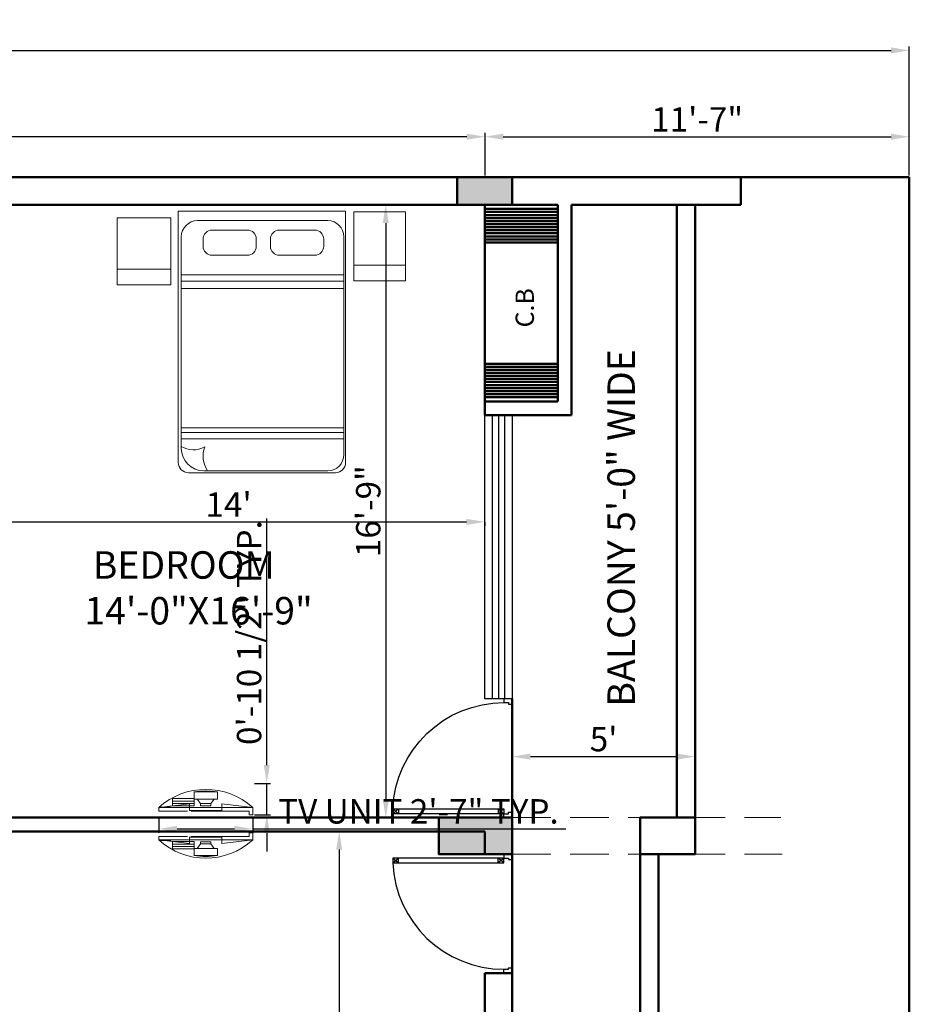
# Model space of a CAD drawing. Units: millimetres. Extents: x 1706 to 5913, y 156 to 1716.
# Tile 5 of 26: x 2351 to 2643, y 573 to 896. Entities that reach past the tile are written whole.
import ezdxf

# ---------------------------------------------------------------- set-up
doc = ezdxf.new("R2010")
doc.units = ezdxf.units.MM
doc.linetypes.add('DASHED', pattern=[19.05, 12.7, -6.35])
for name, color, linetype, lineweight in [('A-ANNO-DIMS', 2, 'Continuous', 18), ('A-AREA-IDEN', 3, 'Continuous', 18), ('A-COLS', 20, 'Continuous', 50), ('A-DOOR', 4, 'Continuous', 25), ('A-FLOR-OVHD', 9, 'DASHED', 18), ('A-FURN', 8, 'Continuous', 18), ('A-GLAZ', 150, 'Continuous', 25), ('A-WALL', 7, 'Continuous', 50)]:
    doc.layers.add(name, color=color, linetype=linetype, lineweight=lineweight)
doc.styles.get("Standard").update_dxf_attribs({"font": 'arial.ttf'})
doc.dimstyles.new('ISO-25', dxfattribs={"dimtxt": 8, "dimasz": 6, "dimexe": 1.25, "dimexo": 0.625, "dimtad": 1, "dimdec": 0, "dimlunit": 3, "dimtxsty": 'Standard', "dimcen": 2.5, "dimadec": 0, "dimazin": 0, "dimtfac": 1, "dimtdec": 0, "dimtmove": 0, "dimatfit": 3, "dimfxl": 1, "dimarcsym": 0})

# ---------------------------------------------------------------- blocks, each defined once
blk = doc.blocks.new('Puerta 01')
for p, q in [((-0.7745, -0.0264), (-0.7368, -0.0584)), ((-0.7745, -0.0584), (-0.7368, -0.0264)), ((-0.7368, -0.0584), (-0.7368, -0.0264)), ((-0.028, -0.0584), (-0.0657, -0.0264)), ((-0.028, -0.0264), (-0.0657, -0.0584)), ((-0.0657, -0.0584), (-0.0657, -0.0264))]:
    blk.add_line(p, q)
for points in [[(-0.028, 0), (-0.028, -0.0264), (0.004, -0.0264), (0.004, -0.036), (0.028, -0.036), (0.028, 0)], [(-0.028, -0.0264), (-0.7745, -0.0264), (-0.7745, -0.0584), (-0.028, -0.0584)], [(0.004, -0.7736), (0.004, -0.764), (0.028, -0.764), (0.028, -0.8), (-0.028, -0.8), (-0.028, -0.7736)]]:
    blk.add_lwpolyline(points, close=True)
blk.add_arc((-0.028, -0.0264), 0.7472, 182.45453, 270)
blk = doc.blocks.new('A$C4AB4758D')
for p, q in [((0.4893, 2.0897), (0.4893, 0.0816)), ((1.8273, 2.0897), (0.4893, 2.0897)), ((1.8273, 0.0816), (1.8273, 2.0897)), ((2.3044, 2.0857), (1.894, 2.0857)), ((1.894, 2.0857), (2.3073, 2.0857)), ((1.894, 2.0857), (1.894, 1.6591)), ((1.894, 1.5327), (1.894, 2.0857)), ((2.3073, 2.0857), (2.3073, 1.5327)), ((0.4262, 2.0383), (0, 2.0383)), ((0, 2.0383), (0.4293, 2.0383)), ((0, 2.0383), (0, 1.6275)), ((0, 1.5028), (0, 2.0383)), ((0.4293, 2.0383), (0.4293, 1.5028)), ((1.6849, 2.015), (0.6419, 2.015)), ((1.041, 1.9394), (0.7595, 1.9394)), ((1.5798, 1.9394), (1.2983, 1.9394)), ((0.5134, 1.8865), (0.5134, 0.1945)), ((0.6871, 1.8671), (0.6871, 1.8107)), ((1.1133, 1.8107), (1.1133, 1.8671)), ((1.226, 1.8671), (1.226, 1.8107)), ((1.6521, 1.8107), (1.6521, 1.8671)), ((1.8134, 0.1435), (1.8134, 1.8865)), ((0.7595, 1.7384), (1.041, 1.7384)), ((1.2983, 1.7384), (1.5798, 1.7384)), ((1.894, 1.6591), (2.3073, 1.6591)), ((0, 1.6275), (0.4293, 1.6275)), ((0.5134, 1.5815), (1.8134, 1.5815)), ((0.4293, 1.5028), (0, 1.5028)), ((0.5134, 1.5305), (1.8134, 1.5305)), ((2.3073, 1.5327), (1.894, 1.5327)), ((0.5134, 1.4724), (1.8134, 1.4724)), ((0.5134, 0.3597), (1.8134, 0.3597)), ((0.5134, 0.3212), (1.8134, 0.3212)), ((0.5134, 0.2703), (1.8134, 0.2703)), ((0.6929, 0.015), (1.6849, 0.015)), ((0.5709, 0), (1.7457, 0))]:
    blk.add_line(p, q)
for centre, radius, start, end in [((0.6419, 1.8865), 0.1285, 90, 180), ((1.6849, 1.8865), 0.1285, 0, 90), ((0.7595, 1.8671), 0.0723, 90, 180), ((1.041, 1.8671), 0.0723, 0, 90), ((1.2983, 1.8671), 0.0723, 90, 180), ((1.5798, 1.8671), 0.0723, 0, 90), ((0.7595, 1.8107), 0.0723, 180, 270), ((1.041, 1.8107), 0.0723, 270, 0), ((1.2983, 1.8107), 0.0723, 180, 270), ((1.5798, 1.8107), 0.0723, 270, 0), ((0.6086, 0.3595), 0.1773, 237.52255, 301.17051), ((0.6929, 0.1945), 0.1795, 180, 270), ((0.8965, 0.1343), 0.2094, 159.47104, 214.45044), ((0.5709, 0.0816), 0.0816, 180, 270), ((1.6849, 0.1435), 0.1285, 270, 0), ((1.7457, 0.0816), 0.0816, 270, 0)]:
    blk.add_arc(centre, radius, start, end)
blk = doc.blocks.new('tv unit')
for p, q in [((5853, 2588), (5205, 2588)), ((5205, 2392), (5205, 2588)), ((5853, 2392), (5853, 2588)), ((5079, 2257), (4229, 2157)), ((4607, 2403), (5207, 2403)), ((4607, 2203), (4607, 2403)), ((4607, 2337), (5207, 2337)), ((4607, 2269), (5207, 2269)), ((5207, 2203), (4607, 2203)), ((5079, 2077), (5079, 2257)), ((5853, 2392), (5205, 2392)), ((5207, 2403), (5207, 2203)), ((5293, 2392), (5385, 2268)), ((5385, 2268), (5672, 2268)), ((5385, 2268), (5385, 2204)), ((5385, 2204), (5672, 2204)), ((5765, 2392), (5672, 2268)), ((5672, 2268), (5672, 2204)), ((5979, 2257), (6829, 2157)), ((5979, 2077), (5979, 2257)), ((6829, 2157), (4229, 2157)), ((4229, 2157), (4229, 2057)), ((5029, 2057), (4229, 2057)), ((5979, 2077), (5079, 2077)), ((6729, 2057), (5129, 2057)), ((6729, 2057), (6729, 1957)), ((6829, 1957), (6729, 1957)), ((6829, 2157), (6829, 1957))]:
    blk.add_line(p, q)
for points in [[(6829, 2157, 0.386509), (4229, 2157, -2.260033)], [(4242, 2140, -0.414214), (4270, 2168), (4561, 2168)]]:
    blk.add_lwpolyline(points, format="xyb")
blk.add_arc((5529, 609), 2006, 80.6925, 99.3075)
blk = doc.blocks.new('*D134')
at = {"layer": 'A-ANNO-DIMS', "color": 0, "lineweight": -2, "transparency": 16777216}
for p, q in [((2470.92, 835.54), (2470.24, 835.54)), ((2471.49, 829.54), (2471.49, 640.54)), ((2470.92, 634.54), (2470.24, 634.54))]:
    blk.add_line(p, q, dxfattribs=at)
at = {"layer": 'A-ANNO-DIMS', "color": 0, "transparency": 16777216}
for points in [[(2470.49, 829.54), (2472.49, 829.54), (2471.49, 835.54)], [(2470.49, 640.54), (2472.49, 640.54), (2471.49, 634.54)]]:
    blk.add_solid(points, dxfattribs=at)
at = {"layer": 'Defpoints', "color": 0, "transparency": 16777216}
for p in [(2471.55, 835.54), (2471.49, 634.54), (2471.55, 634.54)]:
    blk.add_point(p, dxfattribs=at)
at = {"layer": 'A-ANNO-DIMS', "color": 0, "transparency": 16777216, "insert": (2466.78, 735.04), "char_height": 8, "attachment_point": 5, "rotation": 90}
blk.add_mtext('16\'-9"', dxfattribs=at)
blk = doc.blocks.new('*D135')
at = {"layer": 'A-ANNO-DIMS', "color": 0, "lineweight": -2, "transparency": 16777216}
for p, q in [((2335.94, 731.28), (2335.94, 730.28)), ((2341.94, 731.53), (2497.94, 731.53)), ((2503.94, 731.28), (2503.94, 730.28))]:
    blk.add_line(p, q, dxfattribs=at)
at = {"layer": 'A-ANNO-DIMS', "color": 0, "transparency": 16777216}
for points in [[(2341.94, 732.53), (2341.94, 730.53), (2335.94, 731.53)], [(2497.94, 732.53), (2497.94, 730.53), (2503.94, 731.53)]]:
    blk.add_solid(points, dxfattribs=at)
at = {"layer": 'Defpoints', "color": 0, "transparency": 16777216}
for p in [(2335.94, 731.91), (2503.94, 731.91), (2503.94, 731.53)]:
    blk.add_point(p, dxfattribs=at)
at = {"layer": 'A-ANNO-DIMS', "color": 0, "transparency": 16777216, "insert": (2419.94, 736.17), "char_height": 8, "attachment_point": 5}
blk.add_mtext("14'", dxfattribs=at)
blk = doc.blocks.new('*D140')
at = {"layer": 'A-ANNO-DIMS', "color": 0, "lineweight": -2, "transparency": 16777216}
for p, q in [((2452.75, 630.04), (2457.47, 630.04)), ((2456.22, 624.04), (2456.22, 360.04)), ((2452.75, 354.04), (2457.47, 354.04))]:
    blk.add_line(p, q, dxfattribs=at)
at = {"layer": 'A-ANNO-DIMS', "color": 0, "transparency": 16777216}
for points in [[(2455.22, 624.04), (2457.22, 624.04), (2456.22, 630.04)], [(2455.22, 360.04), (2457.22, 360.04), (2456.22, 354.04)]]:
    blk.add_solid(points, dxfattribs=at)
at = {"layer": 'Defpoints', "color": 0, "transparency": 16777216}
for p in [(2452.12, 630.04), (2452.12, 354.04), (2456.22, 354.04)]:
    blk.add_point(p, dxfattribs=at)
at = {"layer": 'A-ANNO-DIMS', "color": 0, "transparency": 16777216, "insert": (2451.51, 492.04), "char_height": 8, "attachment_point": 5, "rotation": 90}
blk.add_mtext("23'", dxfattribs=at)
blk = doc.blocks.new('*D142')
at = {"layer": 'A-ANNO-DIMS', "color": 0, "lineweight": -2, "transparency": 16777216}
for p, q in [((2512.94, 656.74), (2512.94, 653.3)), ((2572.94, 656.74), (2572.94, 653.3)), ((2518.94, 654.55), (2566.94, 654.55))]:
    blk.add_line(p, q, dxfattribs=at)
at = {"layer": 'A-ANNO-DIMS', "color": 0, "transparency": 16777216}
for points in [[(2518.94, 655.55), (2518.94, 653.55), (2512.94, 654.55)], [(2566.94, 655.55), (2566.94, 653.55), (2572.94, 654.55)]]:
    blk.add_solid(points, dxfattribs=at)
at = {"layer": 'Defpoints', "color": 0, "transparency": 16777216}
for p in [(2512.94, 657.36), (2572.94, 657.36), (2572.94, 654.55)]:
    blk.add_point(p, dxfattribs=at)
at = {"layer": 'A-ANNO-DIMS', "color": 0, "transparency": 16777216, "insert": (2542.94, 659.25), "char_height": 8, "attachment_point": 5}
blk.add_mtext("5'", dxfattribs=at)
blk = doc.blocks.new('*D121')
at = {"layer": 'A-ANNO-DIMS', "color": 0, "lineweight": -2, "transparency": 16777216}
for p, q in [((1801.94, 845.16), (1801.94, 859.08)), ((2504.05, 845.16), (2504.05, 859.08)), ((2498.05, 857.83), (1807.94, 857.83))]:
    blk.add_line(p, q, dxfattribs=at)
at = {"layer": 'A-ANNO-DIMS', "color": 0, "transparency": 16777216}
for points in [[(1807.94, 858.83), (1807.94, 856.83), (1801.94, 857.83)], [(2498.05, 858.83), (2498.05, 856.83), (2504.05, 857.83)]]:
    blk.add_solid(points, dxfattribs=at)
at = {"layer": 'Defpoints', "color": 0, "transparency": 16777216}
for p in [(1801.94, 857.83), (1801.94, 844.54), (2504.05, 844.54)]:
    blk.add_point(p, dxfattribs=at)
at = {"layer": 'A-ANNO-DIMS', "color": 0, "transparency": 16777216, "insert": (2153, 862.54), "char_height": 8, "attachment_point": 5}
blk.add_mtext('58\'-6"', dxfattribs=at)
blk = doc.blocks.new('*D122')
at = {"layer": 'A-ANNO-DIMS', "color": 0, "lineweight": -2, "transparency": 16777216}
for p, q in [((2504.05, 845.16), (2504.05, 859.08)), ((2643.23, 845.16), (2643.23, 859.08)), ((2510.05, 857.83), (2637.23, 857.83))]:
    blk.add_line(p, q, dxfattribs=at)
at = {"layer": 'A-ANNO-DIMS', "color": 0, "transparency": 16777216}
for points in [[(2510.05, 858.83), (2510.05, 856.83), (2504.05, 857.83)], [(2637.23, 858.83), (2637.23, 856.83), (2643.23, 857.83)]]:
    blk.add_solid(points, dxfattribs=at)
at = {"layer": 'Defpoints', "color": 0, "transparency": 16777216}
for p in [(2643.23, 857.83), (2504.05, 844.54), (2643.23, 844.54)]:
    blk.add_point(p, dxfattribs=at)
at = {"layer": 'A-ANNO-DIMS', "color": 0, "transparency": 16777216, "insert": (2573.64, 862.47), "char_height": 8, "attachment_point": 5}
blk.add_mtext('11\'-7"', dxfattribs=at)
blk = doc.blocks.new('*D123')
at = {"layer": 'A-ANNO-DIMS', "color": 0, "lineweight": -2, "transparency": 16777216}
for p, q in [((1747.94, 845.16), (1747.94, 887.39)), ((1753.94, 886.14), (2637.23, 886.14)), ((2643.23, 845.16), (2643.23, 887.39))]:
    blk.add_line(p, q, dxfattribs=at)
at = {"layer": 'A-ANNO-DIMS', "color": 0, "transparency": 16777216}
for points in [[(1753.94, 887.14), (1753.94, 885.14), (1747.94, 886.14)], [(2637.23, 887.14), (2637.23, 885.14), (2643.23, 886.14)]]:
    blk.add_solid(points, dxfattribs=at)
at = {"layer": 'Defpoints', "color": 0, "transparency": 16777216}
for p in [(2643.23, 886.14), (1747.94, 844.54), (2643.23, 844.54)]:
    blk.add_point(p, dxfattribs=at)
at = {"layer": 'A-ANNO-DIMS', "color": 0, "transparency": 16777216, "insert": (2195.59, 890.76), "char_height": 8, "attachment_point": 5}
blk.add_mtext('74\'-7"', dxfattribs=at)
blk = doc.blocks.new('*D227')
at = {"layer": 'A-ANNO-DIMS', "color": 0, "lineweight": -2, "transparency": 16777216}
for p, q in [((2397.02, 634.85), (2397.02, 629.6)), ((2427.83, 634.85), (2427.83, 629.6)), ((2403.02, 630.85), (2421.83, 630.85)), ((2427.83, 630.85), (2530.61, 630.85))]:
    blk.add_line(p, q, dxfattribs=at)
at = {"layer": 'A-ANNO-DIMS', "color": 0, "transparency": 16777216}
for points in [[(2403.02, 631.85), (2403.02, 629.85), (2397.02, 630.85)], [(2421.83, 631.85), (2421.83, 629.85), (2427.83, 630.85)]]:
    blk.add_solid(points, dxfattribs=at)
at = {"layer": 'Defpoints', "color": 0, "transparency": 16777216}
for p in [(2397.02, 635.47), (2427.83, 635.47), (2427.83, 630.85)]:
    blk.add_point(p, dxfattribs=at)
at = {"layer": 'A-ANNO-DIMS', "color": 0, "transparency": 16777216, "insert": (2482.22, 635.56), "char_height": 8, "attachment_point": 5}
blk.add_mtext('TV UNIT 2\'-7" TYP.', dxfattribs=at)
blk = doc.blocks.new('*D228')
at = {"layer": 'A-ANNO-DIMS', "color": 0, "lineweight": -2, "transparency": 16777216}
for p, q in [((2432.46, 651.78), (2432.46, 732.65)), ((2428.46, 645.78), (2433.71, 645.78)), ((2432.46, 635.47), (2432.46, 645.78)), ((2428.46, 635.47), (2433.71, 635.47)), ((2432.46, 629.47), (2432.46, 623.47))]:
    blk.add_line(p, q, dxfattribs=at)
at = {"layer": 'A-ANNO-DIMS', "color": 0, "transparency": 16777216}
for points in [[(2431.46, 651.78), (2433.46, 651.78), (2432.46, 645.78)], [(2431.46, 629.47), (2433.46, 629.47), (2432.46, 635.47)]]:
    blk.add_solid(points, dxfattribs=at)
at = {"layer": 'Defpoints', "color": 0, "transparency": 16777216}
for p in [(2427.83, 645.78), (2432.46, 645.78), (2427.83, 635.47)]:
    blk.add_point(p, dxfattribs=at)
at = {"layer": 'A-ANNO-DIMS', "color": 0, "transparency": 16777216, "insert": (2427.69, 695.22), "char_height": 8, "attachment_point": 5, "rotation": 90}
blk.add_mtext('0\'-10 1/2" TYP.', dxfattribs=at)

msp = doc.modelspace()

# ---------------------------------------------------------------- hatches: boundary and pattern name
at = {"layer": 'A-COLS'}
h = msp.add_hatch(color=256, dxfattribs=at)
h.dxf.hatch_style = 1
h.paths.add_polyline_path([(2512.94, 844.54), (2494.94, 844.54), (2494.94, 835.54), (2512.94, 835.54)])
h = msp.add_hatch(color=256, dxfattribs=at)
h.dxf.hatch_style = 1
h.paths.add_polyline_path([(2512.94, 634.54), (2488.94, 634.54), (2488.94, 622.54), (2512.94, 622.54)])

# ---------------------------------------------------------------- linework, layer by layer
msp.add_lwpolyline([(2513.16, 844.54), (2494.94, 844.54), (2494.94, 835.54), (2512.94, 835.54), (2512.94, 844.54)], dxfattribs=at)
msp.add_lwpolyline([(2488.94, 634.54), (2512.94, 634.54), (2512.94, 622.54), (2488.94, 622.54)], close=True, dxfattribs=at)
at = {"layer": 'A-FLOR-OVHD'}
for p, q in [((2512.94, 634.54), (2601.08, 634.54)), ((2512.94, 622.54), (2601.57, 622.54))]:
    msp.add_line(p, q, dxfattribs=at)
at = {"layer": 'A-GLAZ'}
for p, q in [((2506.44, 766.54), (2506.44, 673.54)), ((2508.44, 766.54), (2508.44, 673.54)), ((2510.44, 766.54), (2510.44, 673.54))]:
    msp.add_line(p, q, dxfattribs=at)
msp.add_lwpolyline([(2503.94, 766.54), (2512.94, 766.54), (2512.94, 673.54), (2503.94, 673.54)], close=True, dxfattribs=at)
at = {"layer": 'A-WALL'}
for p, q in [((1773.44, 844.54), (2587.94, 844.54)), ((2512.94, 844.54), (2512.94, 835.54)), ((2512.94, 844.54), (2512.94, 835.54)), ((2512.94, 835.54), (2512.94, 844.54)), ((2587.94, 844.54), (2587.94, 835.54)), ((2587.94, 844.54), (2619.23, 844.54)), ((2619.23, 844.54), (2643.23, 844.54)), ((2643.23, 844.54), (2643.23, 321.04)), ((2259.44, 835.54), (2527.94, 835.54)), ((2503.94, 766.54), (2503.94, 835.54)), ((2503.94, 834.16), (2527.94, 834.16)), ((2503.94, 833.16), (2527.94, 833.16)), ((2527.94, 835.54), (2527.94, 771.04)), ((2532.44, 835.54), (2532.44, 766.54)), ((2532.44, 835.54), (2587.94, 835.54)), ((2566.94, 835.54), (2566.94, 634.54)), ((2572.94, 835.54), (2572.94, 634.54)), ((2503.94, 832.16), (2527.94, 832.16)), ((2503.94, 831.16), (2527.94, 831.16)), ((2503.94, 830.16), (2527.94, 830.16)), ((2503.94, 829.16), (2527.94, 829.16)), ((2503.94, 828.16), (2527.94, 828.16)), ((2503.94, 827.16), (2527.94, 827.16)), ((2503.94, 826.16), (2527.94, 826.16)), ((2503.94, 825.16), (2527.94, 825.16)), ((2503.94, 824.16), (2527.94, 824.16)), ((2503.94, 823.16), (2527.94, 823.16)), ((2503.94, 783.41), (2527.94, 783.41)), ((2503.94, 782.41), (2527.94, 782.41)), ((2503.94, 781.41), (2527.94, 781.41)), ((2503.94, 780.41), (2527.94, 780.41)), ((2503.94, 779.41), (2527.94, 779.41)), ((2503.94, 778.41), (2527.94, 778.41)), ((2503.94, 777.41), (2527.94, 777.41)), ((2503.94, 776.41), (2527.94, 776.41)), ((2503.94, 775.41), (2527.94, 775.41)), ((2503.94, 774.41), (2527.94, 774.41)), ((2503.94, 773.41), (2527.94, 773.41)), ((2503.94, 772.41), (2527.94, 772.41)), ((2503.94, 771.04), (2527.94, 771.04)), ((2503.94, 766.54), (2532.44, 766.54)), ((2512.94, 673.54), (2512.94, 634.54)), ((2307.44, 634.54), (2512.94, 634.54)), ((2512.94, 634.54), (2512.94, 622.54)), ((2302.94, 630.04), (2503.94, 630.04)), ((2503.94, 630.04), (2503.94, 622.54)), ((2512.94, 622.54), (2503.94, 622.54)), ((2512.94, 622.54), (2512.94, 583.54)), ((2554.94, 622.54), (2554.94, 354.04)), ((2560.94, 622.54), (2560.94, 354.04)), ((2503.94, 583.54), (2503.94, 526.54)), ((2512.94, 583.54), (2503.94, 583.54)), ((2512.94, 583.54), (2512.94, 526.54))]:
    msp.add_line(p, q, dxfattribs=at)
msp.add_lwpolyline([(2572.94, 634.54), (2554.94, 634.54), (2554.94, 622.54), (2572.94, 622.54)], close=True, dxfattribs=at)

# ---------------------------------------------------------------- block references
at = {"layer": 'A-DOOR', "xscale": -48.75000000000287, "yscale": 48.75000000000287, "zscale": 48.75000000000287, "rotation": 180}
msp.add_blockref('Puerta 01', (2511.58, 634.54), dxfattribs=at)
at = {"layer": 'A-DOOR', "xscale": 48.75000000000287, "yscale": 48.75000000000287, "zscale": 48.75000000000287}
msp.add_blockref('Puerta 01', (2511.58, 622.54), dxfattribs=at)
at = {"layer": 'A-FURN'}
for name, p, xscale, yscale, zscale in [('A$C4AB4758D', (2383.36, 747.66), 41.02055920967828, 41.02055920967828, 41.02055920967828), ('tv unit', (2346.9, 612.28), 0.0118512648876472, 0.0118512648876472, 0.0118512648876472)]:
    msp.add_blockref(name, p, dxfattribs=dict(at, xscale=xscale, yscale=yscale, zscale=zscale))
at = {"layer": 'A-FURN', "xscale": -0.0118512648876472, "yscale": 0.0118512648876472, "zscale": 0.0118512648876472, "rotation": 180}
msp.add_blockref('tv unit', (2346.9, 652.77), dxfattribs=at)

# ---------------------------------------------------------------- texts
at = {"layer": 'A-AREA-IDEN', "attachment_point": 1, "rotation": 90}
for s, width, insert, char_height in [('     C.B', 33.9892, (2514.09, 786.12), 6), ('    BALCONY 5\'-0" WIDE', 166.3136, (2544.21, 659.94), 9)]:
    msp.add_mtext_dynamic_manual_height_columns(s, width=width, gutter_width=12.5, heights=[0], dxfattribs=dict(at, insert=insert, char_height=char_height))
at = {"layer": 'A-AREA-IDEN', "insert": (2369.87, 721.89), "char_height": 9, "attachment_point": 1}
msp.add_mtext_dynamic_manual_height_columns('  BEDROOM\\P 14\'-0"X16\'-9"', width=91.0711, gutter_width=12.5, heights=[0], dxfattribs=at)

# ---------------------------------------------------------------- dimensions: what is measured, and where the dimension line sits
at = {"layer": 'A-ANNO-DIMS'}
for base, p1, p2, picture, middle in [((2643.23, 886.14), (1747.94, 844.54), (2643.23, 844.54), '*D123', (2195.59, 890.76)), ((1801.94, 857.83), (2504.05, 844.54), (1801.94, 844.54), '*D121', (2153, 862.54)), ((2643.23, 857.83), (2504.05, 844.54), (2643.23, 844.54), '*D122', (2573.64, 862.47)), ((2503.94, 731.53), (2335.94, 731.91), (2503.94, 731.91), '*D135', (2419.94, 736.17)), ((2572.94, 654.55), (2512.94, 657.36), (2572.94, 657.36), '*D142', (2542.94, 659.25))]:
    dim = msp.add_linear_dim(base=base, p1=p1, p2=p2, dimstyle='ISO-25', override={"dimclrd": 0, "dimclre": 0, "dimclrt": 0}, dxfattribs=at)
    dim.commit()
    dim.dimension.update_dxf_attribs({"geometry": picture, "text_midpoint": middle})
for base, p1, p2, picture, middle in [((2471.49, 634.54), (2471.55, 835.54), (2471.55, 634.54), '*D134', (2466.78, 735.04)), ((2456.22, 354.04), (2452.12, 630.04), (2452.12, 354.04), '*D140', (2451.51, 492.04))]:
    dim = msp.add_linear_dim(base=base, p1=p1, p2=p2, angle=90, dimstyle='ISO-25', override={"dimclrd": 0, "dimclre": 0, "dimclrt": 0}, dxfattribs=at)
    dim.commit()
    dim.dimension.update_dxf_attribs({"geometry": picture, "text_midpoint": middle})
dim = msp.add_linear_dim(base=(2432.46, 645.78), p1=(2427.83, 635.47), p2=(2427.83, 645.78), angle=90, text='<> TYP.', dimstyle='ISO-25', override={"dimdec": 1, "dimrnd": 0, "dimzin": 1, "dimlunit": 4, "dimfrac": 2}, dxfattribs=at)
dim.commit()
dim.dimension.update_dxf_attribs({"geometry": '*D228', "text_midpoint": (2427.69, 695.22)})
dim = msp.add_linear_dim(base=(2427.83, 630.85), p1=(2397.02, 635.47), p2=(2427.83, 635.47), text='TV UNIT <> TYP.', dimstyle='ISO-25', override={"dimdec": 1, "dimrnd": 0, "dimzin": 1, "dimlunit": 4, "dimfrac": 2}, dxfattribs=at)
dim.commit()
dim.dimension.update_dxf_attribs({"geometry": '*D227', "text_midpoint": (2482.22, 635.56)})

doc.saveas('drawing.dxf')
